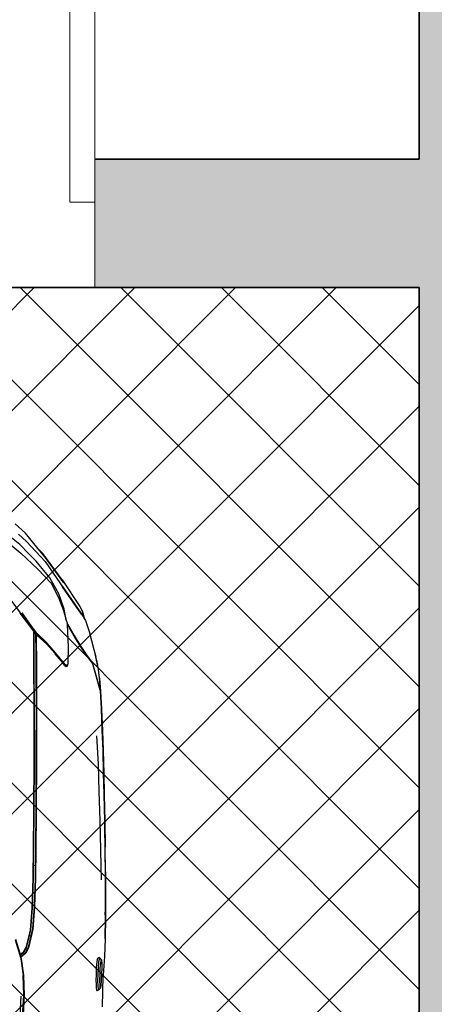
# Model space of a CAD drawing. Units: inches. Extents: x 2167 to 2589, y 1680 to 2489.
# Tile 29 of 38: x 2389 to 2419, y 1796 to 1865. Entities that reach past the tile are written whole.
import ezdxf

# ---------------------------------------------------------------- set-up
doc = ezdxf.new("R2010")
doc.units = ezdxf.units.IN
doc.header["$MEASUREMENT"] = 0
doc.layers.get('0').update_dxf_attribs({"color": 250})
for name, color, linetype, lineweight in [('A-DOOR', 4, 'Continuous', 18), ('A-WALL-PATT', 250, 'Continuous', 13), ('C-PRKG-VEHS', 8, 'Continuous', 13), ('L-PVMT-PATT', 252, 'Continuous', 13), ('walls', 7, 'Continuous', 35)]:
    doc.layers.add(name, color=color, linetype=linetype, lineweight=lineweight)
doc.layers.add('Edges', color=250, linetype='Continuous')

# ---------------------------------------------------------------- blocks, each defined once
blk = doc.blocks.new('*U2')
for p, q in [((0, 0), (0, -6)), ((40, 0), (40, -6))]:
    blk.add_line(p, q)
blk.add_lwpolyline([(0, 0), (0, 40), (1.75, 40), (1.75, 0)], close=True)
blk.add_arc((0, 0), 40, 0, 90)
blk = doc.blocks.new('Nissan Qashqai pl')
at = {"layer": 'Edges'}
for p, q in [((7.7673, 12.7961), (7.8058, 12.8055)), ((7.8087, 12.8062), (7.7848, 12.8012)), ((7.8676, 12.8123), (7.7998, 12.7928)), ((7.8012, 12.7929), (7.8681, 12.8121)), ((7.8106, 12.8065), (7.8087, 12.8062)), ((7.8106, 12.8065), (7.8107, 12.8065)), ((7.8107, 12.8065), (7.8363, 12.8097)), ((7.8363, 12.8097), (7.8676, 12.8123)), ((7.8363, 12.8097), (7.8381, 12.81)), ((7.8381, 12.81), (7.87, 12.8126)), ((7.8676, 12.8123), (7.8681, 12.8121)), ((7.869, 12.8124), (7.8681, 12.8121)), ((7.9137, 12.815), (7.869, 12.8124)), ((7.87, 12.8126), (7.9151, 12.8152)), ((7.9658, 12.8172), (7.9137, 12.815)), ((7.9151, 12.8152), (7.9668, 12.8174)), ((8.016, 12.8189), (7.9658, 12.8172)), ((7.9668, 12.8174), (8.0168, 12.8191)), ((7.9803, 12.803), (8.05, 12.8066)), ((8.0713, 12.8205), (8.016, 12.8189)), ((8.0168, 12.8191), (8.0718, 12.8207)), ((8.05, 12.8066), (8.1176, 12.8087)), ((8.1249, 12.8218), (8.0713, 12.8205)), ((8.0718, 12.8207), (8.1251, 12.822)), ((8.1176, 12.8087), (8.1888, 12.8107)), ((8.1901, 12.8232), (8.1249, 12.8218)), ((8.1251, 12.822), (8.1902, 12.8233)), ((8.1888, 12.8107), (8.2622, 12.8125)), ((8.2094, 12.8235), (8.1901, 12.8232)), ((8.1902, 12.8233), (8.2543, 12.8243)), ((8.2543, 12.8243), (8.2094, 12.8235)), ((8.2543, 12.8243), (8.2094, 12.8235)), ((8.2544, 12.8242), (8.2094, 12.8235)), ((8.2693, 12.8245), (8.2543, 12.8243)), ((8.3166, 12.8249), (8.2544, 12.8242)), ((8.2622, 12.8125), (8.3356, 12.8141)), ((8.3098, 12.825), (8.2693, 12.8245)), ((8.3159, 12.825), (8.2693, 12.8245)), ((8.3159, 12.825), (8.3098, 12.825)), ((8.3159, 12.825), (8.3163, 12.825)), ((8.3163, 12.825), (8.3657, 12.8252)), ((8.3163, 12.825), (8.3597, 12.8252)), ((8.3764, 12.8251), (8.3166, 12.8249)), ((8.3597, 12.8252), (8.3657, 12.8252)), ((8.3657, 12.8252), (8.3663, 12.8252)), ((8.3663, 12.8252), (8.3747, 12.8252)), ((8.3764, 12.8251), (8.3663, 12.8252)), ((8.3747, 12.8252), (8.3757, 12.8252)), ((8.3757, 12.8252), (8.4282, 12.8249)), ((8.4069, 12.8249), (8.3764, 12.8251)), ((8.4219, 12.8246), (8.4069, 12.8249)), ((8.4292, 12.8248), (8.4069, 12.8249)), ((8.4282, 12.8249), (8.4799, 12.8239)), ((8.4799, 12.8239), (8.4292, 12.8248)), ((8.4799, 12.8239), (8.4811, 12.8239)), ((8.4811, 12.8239), (8.5241, 12.8222)), ((8.5241, 12.8222), (8.5707, 12.8193)), ((8.5287, 12.8112), (8.5269, 12.8082)), ((8.5322, 12.8047), (8.5269, 12.8082)), ((8.5287, 12.8112), (8.5331, 12.815)), ((8.5287, 12.8112), (8.531, 12.8095)), ((8.531, 12.8095), (8.5385, 12.8079)), ((8.5322, 12.8047), (8.5375, 12.8036)), ((8.5347, 12.8159), (8.5331, 12.815)), ((8.5331, 12.815), (8.5346, 12.8138)), ((8.5346, 12.8138), (8.5406, 12.8125)), ((8.5407, 12.8167), (8.5347, 12.8159)), ((8.5385, 12.8079), (8.5518, 12.8066)), ((8.5406, 12.8125), (8.5526, 12.8114)), ((8.5527, 12.8169), (8.5407, 12.8167)), ((8.5518, 12.8066), (8.568, 12.8059)), ((8.5526, 12.8114), (8.5681, 12.8107)), ((8.5682, 12.8164), (8.5527, 12.8169)), ((8.568, 12.8059), (8.5842, 12.8057)), ((8.5681, 12.8107), (8.5836, 12.8104)), ((8.5837, 12.8154), (8.5682, 12.8164)), ((8.5707, 12.8193), (8.5719, 12.8193)), ((8.6489, 12.8179), (8.5719, 12.8193)), ((8.5836, 12.8104), (8.5957, 12.8107)), ((8.5958, 12.8141), (8.5837, 12.8154)), ((8.5842, 12.8057), (8.5974, 12.8061)), ((8.5957, 12.8107), (8.6017, 12.8114)), ((8.6018, 12.8129), (8.5958, 12.8141)), ((8.5974, 12.8061), (8.6049, 12.8069)), ((8.6017, 12.8114), (8.6032, 12.8121)), ((8.6032, 12.8121), (8.6018, 12.8129)), ((8.6073, 12.808), (8.6032, 12.8121)), ((8.6049, 12.8069), (8.6073, 12.808)), ((8.6073, 12.808), (8.6093, 12.804)), ((7.6953, 12.7753), (7.7223, 12.7851)), ((7.7223, 12.7851), (7.7673, 12.7961)), ((7.7673, 12.7961), (7.7848, 12.8012)), ((7.7814, 12.7791), (7.7991, 12.7923)), ((7.7984, 12.7909), (7.7828, 12.7793)), ((7.7835, 12.8007), (7.7835, 12.8007)), ((7.7865, 12.8013), (7.7866, 12.8013)), ((7.7936, 12.8029), (7.7977, 12.8038)), ((7.7976, 12.792), (7.7991, 12.7923)), ((7.8007, 12.7926), (7.7984, 12.7909)), ((7.7991, 12.7923), (7.7998, 12.7928)), ((7.7995, 12.7924), (7.8007, 12.7926)), ((7.8012, 12.7929), (7.8007, 12.7926)), ((8.5375, 12.8036), (8.5513, 12.8023)), ((8.5513, 12.8023), (8.5678, 12.8016)), ((8.5678, 12.8016), (8.5844, 12.8014)), ((8.5844, 12.8014), (8.5921, 12.8016)), ((8.5921, 12.8016), (8.6021, 12.8022)), ((8.6021, 12.8022), (8.6065, 12.8027)), ((8.6065, 12.8027), (8.6093, 12.804)), ((7.5946, 12.718), (7.6608, 12.7617)), ((7.6113, 12.7186), (7.6759, 12.7633)), ((7.6799, 12.7658), (7.6125, 12.719)), ((7.6608, 12.7617), (7.6712, 12.7675)), ((7.6712, 12.7675), (7.6721, 12.7679)), ((7.6926, 12.7737), (7.6721, 12.7679)), ((7.6759, 12.7633), (7.6793, 12.7657)), ((7.6911, 12.7728), (7.6774, 12.7688)), ((7.6793, 12.7657), (7.6802, 12.766)), ((7.6799, 12.7658), (7.6802, 12.766)), ((7.6802, 12.766), (7.6809, 12.7664)), ((7.6809, 12.7664), (7.6911, 12.7728)), ((7.6911, 12.7728), (7.6926, 12.7737)), ((7.6926, 12.7737), (7.6953, 12.7753)), ((7.7325, 12.7476), (7.7591, 12.7641)), ((7.7606, 12.7644), (7.7341, 12.7478)), ((7.7591, 12.7641), (7.7814, 12.7791)), ((7.7828, 12.7793), (7.7606, 12.7644)), ((7.7038, 12.731), (7.7325, 12.7476)), ((7.7048, 12.7302), (7.7608, 12.7329)), ((7.7341, 12.7478), (7.7056, 12.7314)), ((7.7608, 12.7329), (7.8014, 12.7318)), ((7.7688, 12.7328), (7.7688, 12.734)), ((7.8014, 12.7318), (7.8022, 12.7316)), ((7.8022, 12.7316), (7.8037, 12.7315)), ((7.8022, 12.7316), (7.8072, 12.73)), ((7.5946, 12.718), (7.5304, 12.6704)), ((7.6024, 12.7221), (7.5387, 12.6759)), ((7.5501, 12.6757), (7.6051, 12.7139)), ((7.6295, 12.7097), (7.59, 12.6877)), ((7.6032, 12.6908), (7.6386, 12.7089)), ((7.6051, 12.7139), (7.6113, 12.7186)), ((7.6051, 12.7139), (7.6111, 12.7181)), ((7.6118, 12.7186), (7.6111, 12.7181)), ((7.6125, 12.719), (7.6118, 12.7186)), ((7.667, 12.723), (7.6295, 12.7097)), ((7.6386, 12.7089), (7.6708, 12.7217)), ((7.6949, 12.7283), (7.667, 12.723)), ((7.6708, 12.7217), (7.6949, 12.7283)), ((7.6949, 12.7283), (7.701, 12.73)), ((7.701, 12.73), (7.7024, 12.7301)), ((7.7024, 12.7301), (7.7038, 12.731)), ((7.7024, 12.7301), (7.7034, 12.7301)), ((7.7056, 12.7314), (7.7034, 12.7301)), ((7.7034, 12.7301), (7.7048, 12.7302)), ((7.7058, 12.7308), (7.7048, 12.7302)), ((7.7938, 12.7171), (7.7748, 12.7018)), ((7.7959, 12.7161), (7.7772, 12.7011)), ((7.8045, 12.7263), (7.7938, 12.7171)), ((7.8062, 12.725), (7.7959, 12.7161)), ((7.8037, 12.7315), (7.8096, 12.7294)), ((7.8072, 12.73), (7.8045, 12.7263)), ((7.8062, 12.725), (7.8087, 12.7283)), ((7.8066, 12.7254), (7.8062, 12.725)), ((7.8096, 12.7294), (7.8066, 12.7254)), ((7.8072, 12.73), (7.8087, 12.7283)), ((7.59, 12.6877), (7.5492, 12.654)), ((7.5687, 12.6579), (7.6032, 12.6908)), ((7.7748, 12.7018), (7.7507, 12.6803)), ((7.753, 12.6794), (7.776, 12.6999)), ((7.776, 12.6999), (7.7539, 12.68)), ((7.7772, 12.7011), (7.776, 12.6999)), ((7.5184, 12.6591), (7.4801, 12.6274)), ((7.5501, 12.6757), (7.5001, 12.6302)), ((7.5387, 12.6759), (7.5184, 12.6591)), ((7.5184, 12.6591), (7.5304, 12.6704)), ((7.7261, 12.6543), (7.7507, 12.6803)), ((7.753, 12.6794), (7.7281, 12.6524)), ((7.7507, 12.6803), (7.7286, 12.6561)), ((7.7539, 12.68), (7.7324, 12.6565)), ((7.531, 12.6359), (7.5081, 12.6131)), ((7.5289, 12.6158), (7.5687, 12.6579)), ((7.531, 12.6359), (7.5301, 12.6353)), ((7.5492, 12.654), (7.531, 12.6359)), ((7.7261, 12.6543), (7.6762, 12.6186)), ((7.6762, 12.6186), (7.7233, 12.6514)), ((7.6771, 12.6135), (7.7215, 12.6473)), ((7.7215, 12.6473), (7.7221, 12.6478)), ((7.7232, 12.6486), (7.7221, 12.6478)), ((7.7281, 12.6524), (7.7232, 12.6486)), ((7.7245, 12.6486), (7.7232, 12.6486)), ((7.7267, 12.6539), (7.7233, 12.6514)), ((7.7261, 12.6476), (7.7238, 12.6476)), ((7.7294, 12.6487), (7.7245, 12.6486)), ((7.7279, 12.6477), (7.7261, 12.6476)), ((7.7286, 12.6561), (7.7267, 12.6539)), ((7.8048, 12.6483), (7.7279, 12.6477)), ((7.7299, 12.6537), (7.7281, 12.6524)), ((7.7281, 12.6524), (7.7349, 12.6524)), ((7.731, 12.6487), (7.7294, 12.6487)), ((7.7324, 12.6565), (7.7299, 12.6537)), ((7.7299, 12.6537), (7.7334, 12.6537)), ((7.764, 12.6489), (7.731, 12.6487)), ((7.7334, 12.6537), (7.8083, 12.6544)), ((7.7349, 12.6524), (7.768, 12.6527)), ((7.7662, 12.6489), (7.764, 12.6489)), ((7.7811, 12.649), (7.7662, 12.6489)), ((7.768, 12.6527), (7.7692, 12.6527)), ((7.7692, 12.6527), (7.7844, 12.6528)), ((7.7822, 12.649), (7.7811, 12.649)), ((7.8057, 12.6491), (7.7822, 12.649)), ((7.7844, 12.6528), (7.8078, 12.653)), ((7.9014, 12.6487), (7.8048, 12.6483)), ((7.8233, 12.6492), (7.8057, 12.6491)), ((7.8078, 12.653), (7.8233, 12.6531)), ((7.8083, 12.6544), (7.904, 12.6547)), ((7.8233, 12.6531), (7.9036, 12.6534)), ((7.902, 12.6495), (7.8233, 12.6492)), ((8.0273, 12.6485), (7.9014, 12.6487)), ((8.0275, 12.6493), (7.902, 12.6495)), ((7.9036, 12.6534), (8.0275, 12.6533)), ((7.904, 12.6547), (8.0276, 12.6545)), ((8.1753, 12.6479), (8.0273, 12.6485)), ((8.0275, 12.6533), (8.1755, 12.6527)), ((8.1754, 12.6487), (8.0275, 12.6493)), ((8.0276, 12.6545), (8.1753, 12.6539)), ((8.1753, 12.6539), (8.3324, 12.6521)), ((8.3318, 12.6462), (8.1753, 12.6479)), ((8.3002, 12.6474), (8.1754, 12.6487)), ((8.1755, 12.6527), (8.3005, 12.6514)), ((8.3005, 12.6514), (8.3002, 12.6474)), ((8.332, 12.6471), (8.3002, 12.6474)), ((8.3005, 12.6514), (8.3324, 12.651)), ((8.4049, 12.6437), (8.3318, 12.6462)), ((8.4042, 12.6447), (8.332, 12.6471)), ((8.3324, 12.6521), (8.4022, 12.6498)), ((8.3324, 12.651), (8.4014, 12.6488)), ((8.4014, 12.6488), (8.4559, 12.6451)), ((8.4022, 12.6498), (8.4571, 12.6459)), ((8.4588, 12.6405), (8.4042, 12.6447)), ((8.4595, 12.6395), (8.4049, 12.6437)), ((8.4559, 12.6451), (8.4736, 12.6409)), ((8.4571, 12.6459), (8.5029, 12.635)), ((8.4729, 12.6372), (8.4588, 12.6405)), ((8.5025, 12.6293), (8.4595, 12.6395)), ((8.4729, 12.6372), (8.4736, 12.6409)), ((8.5032, 12.6301), (8.4729, 12.6372)), ((8.4736, 12.6409), (8.5018, 12.6344)), ((8.5018, 12.6344), (8.5155, 12.6274)), ((8.5029, 12.635), (8.5163, 12.6279)), ((7.4801, 12.6274), (7.4565, 12.6023)), ((7.5081, 12.6131), (7.4679, 12.5634)), ((7.4827, 12.6103), (7.5001, 12.6302)), ((7.4884, 12.5664), (7.5289, 12.6158)), ((7.5243, 12.6101), (7.5286, 12.6146)), ((7.676, 12.6152), (7.6296, 12.5803)), ((8.4814, 12.6029), (8.5166, 12.6135)), ((8.5216, 12.6139), (8.4838, 12.6027)), ((8.5125, 12.6231), (8.5025, 12.6293)), ((8.5132, 12.624), (8.5032, 12.6301)), ((8.5177, 12.617), (8.5125, 12.6231)), ((8.5132, 12.624), (8.5216, 12.6139)), ((8.5155, 12.6274), (8.5258, 12.6151)), ((8.5163, 12.6279), (8.5237, 12.6189)), ((8.5166, 12.6135), (8.5197, 12.6145)), ((8.5197, 12.6145), (8.5177, 12.617)), ((8.5197, 12.6145), (8.5216, 12.6139)), ((8.5258, 12.6151), (8.5216, 12.6139)), ((8.5237, 12.6189), (8.5259, 12.6162)), ((8.5259, 12.6162), (8.5258, 12.6151)), ((8.5258, 12.6151), (8.5304, 12.6157)), ((8.5259, 12.6162), (8.5294, 12.6167)), ((8.5294, 12.6167), (8.5706, 12.6226)), ((8.5304, 12.6157), (8.5715, 12.6215)), ((8.5304, 12.6157), (8.5304, 12.6157)), ((8.5706, 12.6226), (8.6197, 12.6241)), ((8.6203, 12.6229), (8.5715, 12.6215)), ((8.6197, 12.6241), (8.6683, 12.6215)), ((8.6203, 12.6229), (8.6204, 12.6229)), ((8.6721, 12.6201), (8.6204, 12.6229)), ((8.622, 12.6161), (8.6699, 12.6132))]:
    blk.add_line(p, q, dxfattribs=at)
blk = doc.blocks.new('car')
blk.add_blockref('Nissan Qashqai pl', (-9.7433, -11.9151))
blk = doc.blocks.new('carr')
blk.add_blockref('car', (0.5124, -0.007))

msp = doc.modelspace()

# ---------------------------------------------------------------- hatches: boundary and pattern name
at = {"layer": 'A-WALL-PATT'}
h = msp.add_hatch(color=256, dxfattribs=at)
h.dxf.hatch_style = 1
h.paths.add_polyline_path([(2274.738, 1855.042), (2224.048, 1855.042), (2224.048, 2003.119), (2215.048, 2003.119), (2215.048, 1846.042), (2274.738, 1846.042)])
h.paths.add_polyline_path([(2354.886, 1855.042), (2330.895, 1855.042), (2330.895, 1846.042), (2354.773, 1846.042), (2354.773, 1852.042, -0.01877)])
h.paths.add_polyline_path([(2422.048, 1864.695), (2426.208, 1864.695), (2426.208, 1867.924), (2426.208, 1869.195), (2422.048, 1869.195), (2422.048, 1916.243), (2417.548, 1916.243), (2417.548, 1855.042), (2394.773, 1855.042), (2394.773, 1852.042), (2394.773, 1846.042), (2417.548, 1846.042), (2417.548, 1779.195), (2427.738, 1779.195), (2427.738, 1783.941), (2427.738, 1788.195), (2422.048, 1788.195)])
at = {"layer": 'L-PVMT-PATT'}
h = msp.add_hatch(dxfattribs=at)
h.set_pattern_fill('ANSI37', color=256, scale=40)
h.paths.add_polyline_path([(2417.548, 1783.695), (2417.548, 1846.042), (2239.361, 1846.042), (2239.361, 1687.695), (2369.843, 1687.695), (2369.843, 1696.695), (2375.607, 1696.695), (2416.107, 1696.695), (2417.548, 1696.695)])

# ---------------------------------------------------------------- linework, layer by layer
at = {"layer": 'walls'}
for p, q in [((2417.548, 1916.243), (2417.548, 1855.042)), ((2394.773, 1855.042), (2417.548, 1855.042)), ((2215.048, 1846.042), (2417.548, 1846.042)), ((2417.548, 1846.042), (2417.548, 1779.195))]:
    msp.add_line(p, q, dxfattribs=at)

# ---------------------------------------------------------------- block references
at = {"layer": 'A-DOOR', "xscale": -1}
msp.add_blockref('*U2', (2394.773, 1852.042), dxfattribs=at)
at = {"layer": 'C-PRKG-VEHS', "xscale": 28.42784210623918, "yscale": 28.42784210623918, "zscale": 28.42784210623918, "rotation": 270}
msp.add_blockref('carr', (2369.852, 1779.037), dxfattribs=at)

doc.saveas('drawing.dxf')
